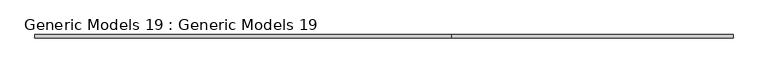
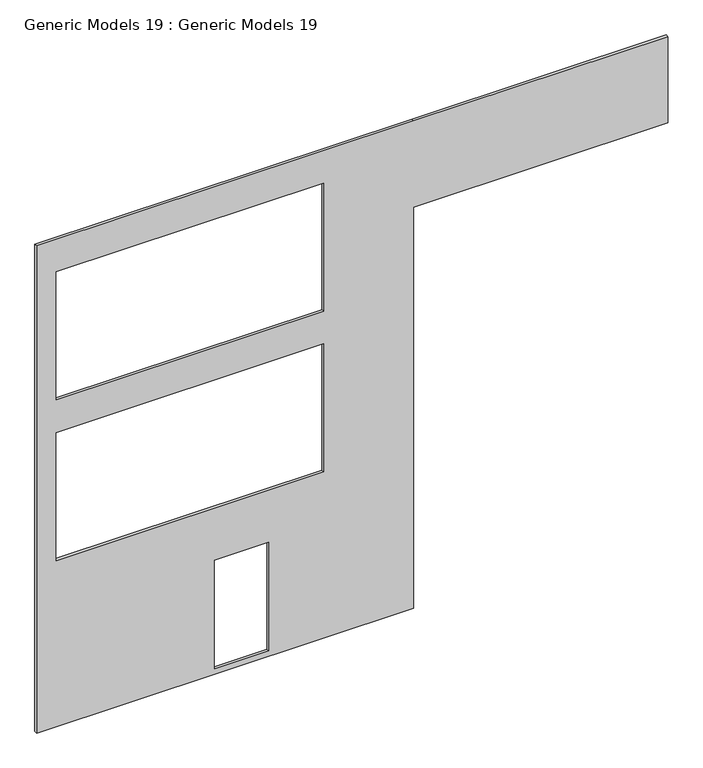
"""IFC4 building model written with IfcOpenShell, lengths in millimetres: proxy geometry, Generic Models 19 : Generic Models 19."""

from ifc_helpers import new_model, si_unit, frame, origin, place, context, project, spatial, polyline, outline, extrude, source, transform, mapped, element, save


def generic_models_19_generic_models_19_d8e6bd8f(model_context):
    return source(origin(), model_context, "Body", "SweptSolid", [
        extrude(outline(polyline([(9448.8, -2677.3781265), (9448.8, -9446.4781265), (203.2, -9446.4781265), (203.2, -2677.3781265), (7810.4767967, -2677.3781265), (7810.4767967, 1894.6218735), (9448.8, 1894.6218735), (9448.8, -2677.3781265)]), holes=[polyline([(8829.7640157, -9090.8781265), (8829.7640157, -4290.2781265), (6400.8, -4290.2781265), (6400.8, -9090.8781265), (8829.7640157, -9090.8781265)]), polyline([(5781.7640157, -9090.8781265), (5781.7640157, -4290.2781265), (3352.8, -4290.2781265), (3352.8, -9090.8781265), (5781.7640157, -9090.8781265)]), polyline([(2362.2, -6246.0781265), (2362.2, -5280.8781265), (304.8, -5280.8781265), (304.8, -6246.0781265), (2362.2, -6246.0781265)])]), frame((0.0, 8336.1857468, 0.0), z_axis=(0.0, 1.0, 0.0), x_axis=(0.0, 0.0, 1.0)), (0.0, 0.0, 1.0), 50.8),
    ])


if __name__ == "__main__":
    model = new_model("IFC4")
    model_context = context("Model", 3, world=origin())
    ifc_project = project(units=[si_unit("LENGTHUNIT", "METRE", prefix="MILLI")], contexts=[model_context])
    site = spatial("IfcSite", under=ifc_project)
    building = spatial("IfcBuilding", under=site)
    placement = place(None, origin())
    generic_models_19_generic_models_19_shape = generic_models_19_generic_models_19_d8e6bd8f(model_context)
    element("IfcBuildingElementProxy", 1, Name="Generic Models 19 : Generic Models 19", ObjectType="Generic Models 19 : Generic Models 19", at=placement, inside=building, context=model_context, shape_type="MappedRepresentation", body=[
        mapped(generic_models_19_generic_models_19_shape, transform((0.0, 0.0, 0.0), x_axis=(1.0, 0.0, 0.0), y_axis=(0.0, 1.0, 0.0), z_axis=(0.0, 0.0, 1.0))),
    ])
    save(model, "model.ifc")
